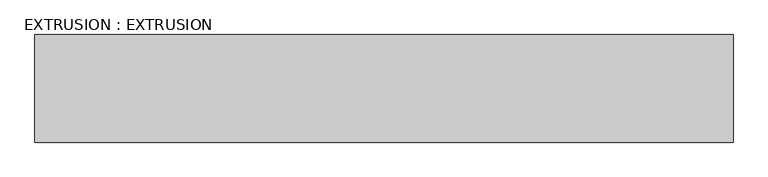
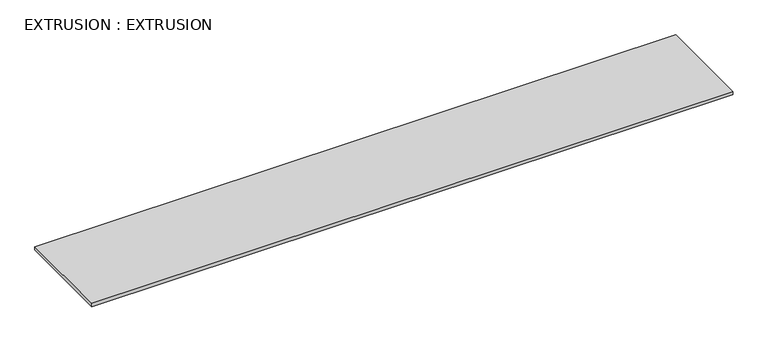
"""IFC4 building model written with IfcOpenShell, lengths in millimetres: proxy geometry, EXTRUSION : EXTRUSION."""

from ifc_helpers import new_model, si_unit, frame, origin, place, context, project, spatial, polyline, outline, extrude, source, transform, mapped, element, save


def extrusion_extrusion_7330b34c(model_context):
    return source(origin(), model_context, "Body", "SweptSolid", [
        extrude(outline(polyline([(10446.7316875, 15280.1035433), (-640.5839017, 15280.1035433), (-640.5839017, 16989.0323212), (10446.7316875, 16989.0323212), (10446.7316875, 15280.1035433)])), frame((0.0, 0.0, -76.2), z_axis=(0.0, 0.0, 1.0), x_axis=(1.0, 0.0, 0.0)), (0.0, 0.0, 1.0), 58.5159536),
    ])


if __name__ == "__main__":
    model = new_model("IFC4")
    model_context = context("Model", 3, world=origin())
    ifc_project = project(units=[si_unit("LENGTHUNIT", "METRE", prefix="MILLI")], contexts=[model_context])
    site = spatial("IfcSite", under=ifc_project)
    building = spatial("IfcBuilding", under=site)
    placement = place(None, origin())
    extrusion_extrusion_shape = extrusion_extrusion_7330b34c(model_context)
    element("IfcBuildingElementProxy", 1, Name="EXTRUSION : EXTRUSION", ObjectType="EXTRUSION : EXTRUSION", at=placement, inside=building, context=model_context, shape_type="MappedRepresentation", body=[
        mapped(extrusion_extrusion_shape, transform((0.0, 0.0, 0.0), x_axis=(1.0, 0.0, 0.0), y_axis=(0.0, 1.0, 0.0), z_axis=(0.0, 0.0, 1.0))),
    ])
    save(model, "model.ifc")
